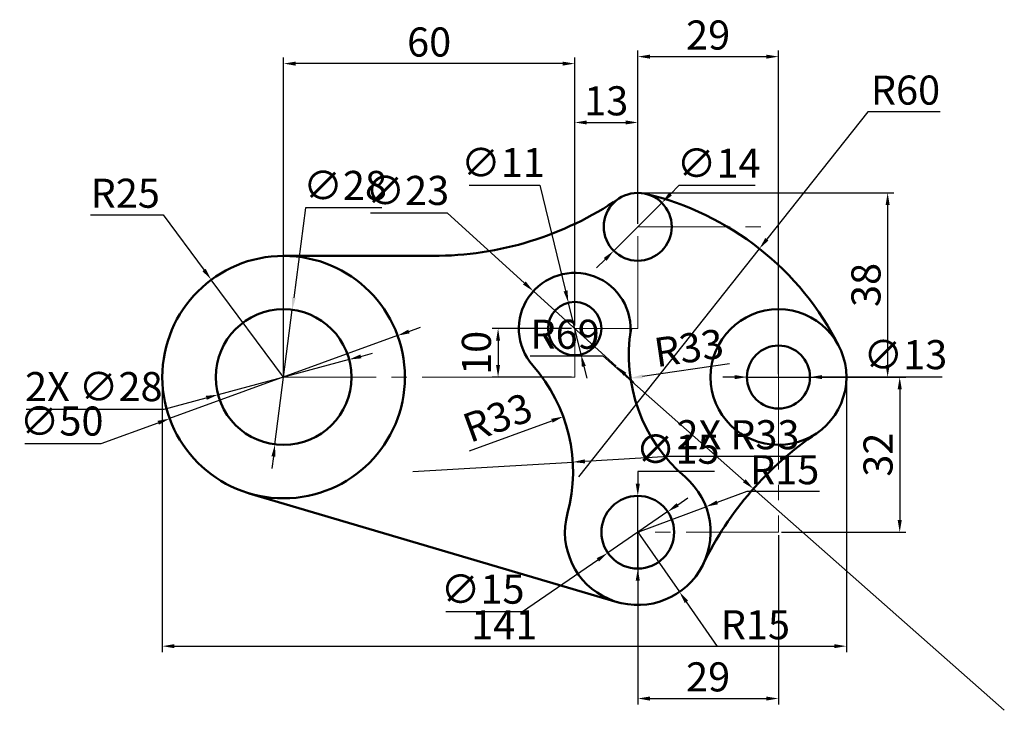
# Model space of a CAD drawing. Units: millimetres. Extents: x 48 to 251, y 61 to 204.
import ezdxf

# ---------------------------------------------------------------- set-up
doc = ezdxf.new("R2010")
doc.units = ezdxf.units.MM
doc.linetypes.add('CENTER2', pattern=[28.575, 19.05, -3.175, 3.175, -3.175])
for name, color, linetype, lineweight in [('M-CNTR', 4, 'CENTER2', 18), ('M-DIMS', 2, 'Continuous', 25), ('M-OUTL', 7, 'Continuous', 50)]:
    doc.layers.add(name, color=color, linetype=linetype, lineweight=lineweight)
doc.styles.get("Standard").update_dxf_attribs({"font": 'arial.ttf'})
doc.dimstyles.new('ISO-25', dxfattribs={"dimtxt": 6, "dimasz": 2.5, "dimexe": 1.25, "dimexo": 0.625, "dimtad": 1, "dimtoh": 1, "dimdec": 0, "dimtxsty": 'Standard', "dimcen": 2.5, "dimadec": 0, "dimazin": 0, "dimtfac": 1, "dimtdec": 0, "dimtmove": 0, "dimatfit": 3, "dimfxl": 1, "dimarcsym": 0})

# ---------------------------------------------------------------- blocks, each defined once
blk = doc.blocks.new('*D1')
at = {"layer": 'Defpoints', "color": 0, "transparency": 16777216}
for p in [(162.88, 140.02), (147.09, 130.02), (162.88, 130.02)]:
    blk.add_point(p, dxfattribs=at)
at = {"layer": 'M-DIMS', "color": 0, "lineweight": -2, "transparency": 16777216}
for p, q in [((162.25, 140.02), (145.84, 140.02)), ((147.09, 137.52), (147.09, 132.52)), ((162.25, 130.02), (145.84, 130.02))]:
    blk.add_line(p, q, dxfattribs=at)
at = {"layer": 'M-DIMS', "color": 0, "transparency": 16777216}
for points in [[(146.67, 137.52), (147.5, 137.52), (147.09, 140.02)], [(146.67, 132.52), (147.5, 132.52), (147.09, 130.02)]]:
    blk.add_solid(points, dxfattribs=at)
at = {"layer": 'M-DIMS', "color": 0, "transparency": 16777216, "insert": (143.4, 135.02), "char_height": 6, "attachment_point": 5, "rotation": 90}
blk.add_mtext('10', dxfattribs=at)
blk = doc.blocks.new('*D2')
at = {"layer": 'Defpoints', "color": 0, "transparency": 16777216}
for p in [(154.36, 147.74), (171.4, 132.29)]:
    blk.add_point(p, dxfattribs=at)
at = {"layer": 'M-DIMS', "color": 0, "lineweight": -2, "transparency": 16777216}
for p, q in [((120.81, 163.89), (136.56, 163.89)), ((136.56, 163.89), (152.51, 149.42)), ((171.4, 132.29), (154.36, 147.74)), ((173.25, 130.61), (175.1, 128.93))]:
    blk.add_line(p, q, dxfattribs=at)
at = {"layer": 'M-DIMS', "color": 0, "transparency": 16777216}
for points in [[(152.79, 149.73), (152.23, 149.11), (154.36, 147.74)], [(173.53, 130.92), (172.97, 130.3), (171.4, 132.29)]]:
    blk.add_solid(points, dxfattribs=at)
at = {"layer": 'M-DIMS', "color": 0, "transparency": 16777216, "insert": (128.37, 167.74), "char_height": 6, "attachment_point": 5}
blk.add_mtext('∅23', dxfattribs=at)
blk = doc.blocks.new('*D3')
at = {"layer": 'Defpoints', "color": 0, "transparency": 16777216}
for p in [(161.58, 145.36), (164.18, 134.67)]:
    blk.add_point(p, dxfattribs=at)
at = {"layer": 'M-DIMS', "color": 0, "lineweight": -2, "transparency": 16777216}
for p, q in [((141.11, 169.62), (155.7, 169.62)), ((155.7, 169.62), (160.99, 147.79)), ((164.18, 134.67), (161.58, 145.36)), ((164.77, 132.24), (165.35, 129.81))]:
    blk.add_line(p, q, dxfattribs=at)
at = {"layer": 'M-DIMS', "color": 0, "transparency": 16777216}
for points in [[(161.4, 147.89), (160.59, 147.69), (161.58, 145.36)], [(165.17, 132.34), (164.36, 132.14), (164.18, 134.67)]]:
    blk.add_solid(points, dxfattribs=at)
at = {"layer": 'M-DIMS', "color": 0, "transparency": 16777216, "insert": (148.09, 173.48), "char_height": 6, "attachment_point": 5}
blk.add_mtext('∅11', dxfattribs=at)
blk = doc.blocks.new('*D4')
at = {"layer": 'Defpoints', "color": 0, "transparency": 16777216}
for p in [(175.88, 182.53), (175.88, 161.02), (162.88, 140.02)]:
    blk.add_point(p, dxfattribs=at)
at = {"layer": 'M-DIMS', "color": 0, "lineweight": -2, "transparency": 16777216}
for p, q in [((162.88, 140.64), (162.88, 183.78)), ((175.88, 161.64), (175.88, 183.78)), ((165.38, 182.53), (173.38, 182.53))]:
    blk.add_line(p, q, dxfattribs=at)
at = {"layer": 'M-DIMS', "color": 0, "transparency": 16777216}
for points in [[(165.38, 182.95), (165.38, 182.12), (162.88, 182.53)], [(173.38, 182.95), (173.38, 182.12), (175.88, 182.53)]]:
    blk.add_solid(points, dxfattribs=at)
at = {"layer": 'M-DIMS', "color": 0, "transparency": 16777216, "insert": (169.38, 186.22), "char_height": 6, "attachment_point": 5}
blk.add_mtext('13', dxfattribs=at)
blk = doc.blocks.new('*D5')
at = {"layer": 'Defpoints', "color": 0, "transparency": 16777216}
for p in [(204.88, 130.02), (204.88, 98.02), (229.87, 98.02)]:
    blk.add_point(p, dxfattribs=at)
at = {"layer": 'M-DIMS', "color": 0, "lineweight": -2, "transparency": 16777216}
for p, q in [((205.5, 130.02), (231.12, 130.02)), ((229.87, 127.52), (229.87, 100.52)), ((205.5, 98.02), (231.12, 98.02))]:
    blk.add_line(p, q, dxfattribs=at)
at = {"layer": 'M-DIMS', "color": 0, "transparency": 16777216}
for points in [[(229.45, 127.52), (230.29, 127.52), (229.87, 130.02)], [(229.45, 100.52), (230.29, 100.52), (229.87, 98.02)]]:
    blk.add_solid(points, dxfattribs=at)
at = {"layer": 'M-DIMS', "color": 0, "transparency": 16777216, "insert": (226.18, 114.02), "char_height": 6, "attachment_point": 5, "rotation": 90}
blk.add_mtext('32', dxfattribs=at)
blk = doc.blocks.new('*D6')
at = {"layer": 'Defpoints', "color": 0, "transparency": 16777216}
for p in [(175.88, 98.02), (204.88, 98.02), (204.88, 63.73)]:
    blk.add_point(p, dxfattribs=at)
at = {"layer": 'M-DIMS', "color": 0, "lineweight": -2, "transparency": 16777216}
for p, q in [((175.88, 97.39), (175.88, 62.48)), ((204.88, 97.39), (204.88, 62.48)), ((178.38, 63.73), (202.38, 63.73))]:
    blk.add_line(p, q, dxfattribs=at)
at = {"layer": 'M-DIMS', "color": 0, "transparency": 16777216}
for points in [[(178.38, 64.14), (178.38, 63.31), (175.88, 63.73)], [(202.38, 64.14), (202.38, 63.31), (204.88, 63.73)]]:
    blk.add_solid(points, dxfattribs=at)
at = {"layer": 'M-DIMS', "color": 0, "transparency": 16777216, "insert": (190.38, 67.42), "char_height": 6, "attachment_point": 5}
blk.add_mtext('29', dxfattribs=at)
blk = doc.blocks.new('*D7')
at = {"layer": 'Defpoints', "color": 0, "transparency": 16777216}
for p in [(182.06, 102.27), (169.7, 93.76)]:
    blk.add_point(p, dxfattribs=at)
at = {"layer": 'M-DIMS', "color": 0, "lineweight": -2, "transparency": 16777216}
for p, q in [((184.12, 103.69), (186.18, 105.11)), ((182.06, 102.27), (169.7, 93.76)), ((152.11, 81.66), (167.64, 92.35)), ((136.32, 81.66), (152.11, 81.66))]:
    blk.add_line(p, q, dxfattribs=at)
at = {"layer": 'M-DIMS', "color": 0, "transparency": 16777216}
for points in [[(183.88, 104.03), (184.35, 103.34), (182.06, 102.27)], [(167.41, 92.69), (167.88, 92), (169.7, 93.76)]]:
    blk.add_solid(points, dxfattribs=at)
at = {"layer": 'M-DIMS', "color": 0, "transparency": 16777216, "insert": (143.9, 85.51), "char_height": 6, "attachment_point": 5}
blk.add_mtext('∅15', dxfattribs=at)
blk = doc.blocks.new('*D8')
at = {"layer": 'Defpoints', "color": 0, "transparency": 16777216}
for p in [(175.88, 98.02), (184.47, 85.72)]:
    blk.add_point(p, dxfattribs=at)
at = {"layer": 'M-DIMS', "color": 0, "lineweight": -2, "transparency": 16777216}
for p, q in [((175.88, 98.02), (184.47, 85.72)), ((192.31, 74.48), (185.9, 83.67)), ((207.31, 74.48), (192.31, 74.48))]:
    blk.add_line(p, q, dxfattribs=at)
at = {"layer": 'M-DIMS', "color": 0, "transparency": 16777216}
blk.add_solid([(186.24, 83.91), (185.56, 83.43), (184.47, 85.72)], dxfattribs=at)
at = {"layer": 'M-DIMS', "color": 0, "transparency": 16777216, "insert": (200.12, 78.17), "char_height": 6, "attachment_point": 5}
blk.add_mtext('R15', dxfattribs=at)
blk = doc.blocks.new('*D9')
at = {"layer": 'Defpoints', "color": 0, "transparency": 16777216}
for p in [(204.88, 196.11), (175.88, 161.02), (204.88, 130.02)]:
    blk.add_point(p, dxfattribs=at)
at = {"layer": 'M-DIMS', "color": 0, "lineweight": -2, "transparency": 16777216}
for p, q in [((175.88, 161.64), (175.88, 197.36)), ((204.88, 130.64), (204.88, 197.36)), ((178.38, 196.11), (202.38, 196.11))]:
    blk.add_line(p, q, dxfattribs=at)
at = {"layer": 'M-DIMS', "color": 0, "transparency": 16777216}
for points in [[(178.38, 196.52), (178.38, 195.69), (175.88, 196.11)], [(202.38, 196.52), (202.38, 195.69), (204.88, 196.11)]]:
    blk.add_solid(points, dxfattribs=at)
at = {"layer": 'M-DIMS', "color": 0, "transparency": 16777216, "insert": (190.38, 199.79), "char_height": 6, "attachment_point": 5}
blk.add_mtext('29', dxfattribs=at)
blk = doc.blocks.new('*D10')
at = {"layer": 'Defpoints', "color": 0, "transparency": 16777216}
for p in [(102.88, 194.67), (162.88, 140.02), (102.88, 130.02)]:
    blk.add_point(p, dxfattribs=at)
at = {"layer": 'M-DIMS', "color": 0, "lineweight": -2, "transparency": 16777216}
for p, q in [((102.88, 130.64), (102.88, 195.92)), ((162.88, 140.64), (162.88, 195.92)), ((160.38, 194.67), (105.38, 194.67))]:
    blk.add_line(p, q, dxfattribs=at)
at = {"layer": 'M-DIMS', "color": 0, "transparency": 16777216}
for points in [[(105.38, 195.08), (105.38, 194.25), (102.88, 194.67)], [(160.38, 195.08), (160.38, 194.25), (162.88, 194.67)]]:
    blk.add_solid(points, dxfattribs=at)
at = {"layer": 'M-DIMS', "color": 0, "transparency": 16777216, "insert": (132.88, 198.35), "char_height": 6, "attachment_point": 5}
blk.add_mtext('60', dxfattribs=at)
blk = doc.blocks.new('*D11')
at = {"layer": 'Defpoints', "color": 0, "transparency": 16777216}
for p in [(87.98, 150.09), (102.88, 130.02)]:
    blk.add_point(p, dxfattribs=at)
at = {"layer": 'M-DIMS', "color": 0, "lineweight": -2, "transparency": 16777216}
for p, q in [((63.05, 163.47), (78.06, 163.47)), ((78.06, 163.47), (86.49, 152.1)), ((102.88, 130.02), (87.98, 150.09))]:
    blk.add_line(p, q, dxfattribs=at)
at = {"layer": 'M-DIMS', "color": 0, "transparency": 16777216}
blk.add_solid([(86.83, 152.35), (86.16, 151.85), (87.98, 150.09)], dxfattribs=at)
at = {"layer": 'M-DIMS', "color": 0, "transparency": 16777216, "insert": (70.24, 167.16), "char_height": 6, "attachment_point": 5}
blk.add_mtext('R25', dxfattribs=at)
blk = doc.blocks.new('*D12')
at = {"layer": 'Defpoints', "color": 0, "transparency": 16777216}
for p in [(104.66, 143.9), (101.1, 116.13)]:
    blk.add_point(p, dxfattribs=at)
at = {"layer": 'M-DIMS', "color": 0, "lineweight": -2, "transparency": 16777216}
for p, q in [((107.36, 164.91), (104.98, 146.38)), ((123.12, 164.91), (107.36, 164.91)), ((101.1, 116.13), (104.66, 143.9)), ((100.78, 113.65), (100.46, 111.17))]:
    blk.add_line(p, q, dxfattribs=at)
at = {"layer": 'M-DIMS', "color": 0, "transparency": 16777216}
for points in [[(104.57, 146.44), (105.39, 146.33), (104.66, 143.9)], [(100.37, 113.7), (101.19, 113.6), (101.1, 116.13)]]:
    blk.add_solid(points, dxfattribs=at)
at = {"layer": 'M-DIMS', "color": 0, "transparency": 16777216, "insert": (115.55, 168.77), "char_height": 6, "attachment_point": 5}
blk.add_mtext('∅28', dxfattribs=at)
blk = doc.blocks.new('*D13')
at = {"layer": 'Defpoints', "color": 0, "transparency": 16777216}
for p in [(160.53, 121.88), (129.54, 110.54)]:
    blk.add_point(p, dxfattribs=at)
at = {"layer": 'M-DIMS', "color": 0, "lineweight": -2, "transparency": 16777216}
blk.add_line((141.2, 114.81), (158.19, 121.02), dxfattribs=at)
at = {"layer": 'M-DIMS', "color": 0, "transparency": 16777216}
blk.add_solid([(158.04, 121.41), (158.33, 120.63), (160.53, 121.88)], dxfattribs=at)
at = {"layer": 'M-DIMS', "color": 0, "transparency": 16777216, "insert": (147.25, 120.95), "char_height": 6, "attachment_point": 5, "rotation": 20.0942}
blk.add_mtext('R33', dxfattribs=at)
blk = doc.blocks.new('*D14')
at = {"layer": 'Defpoints', "color": 0, "transparency": 16777216}
for p in [(207.04, 134.53), (174.38, 129.79)]:
    blk.add_point(p, dxfattribs=at)
at = {"layer": 'M-DIMS', "color": 0, "lineweight": -2, "transparency": 16777216}
blk.add_line((194.76, 132.75), (176.86, 130.15), dxfattribs=at)
at = {"layer": 'M-DIMS', "color": 0, "transparency": 16777216}
blk.add_solid([(176.8, 130.57), (176.92, 129.74), (174.38, 129.79)], dxfattribs=at)
at = {"layer": 'M-DIMS', "color": 0, "transparency": 16777216, "insert": (186.51, 135.28), "char_height": 6, "attachment_point": 5, "rotation": 8.2467}
blk.add_mtext('R33', dxfattribs=at)
blk = doc.blocks.new('*D15')
at = {"layer": 'Defpoints', "color": 0, "transparency": 16777216}
for p in [(77.88, 130.02), (218.88, 130.02), (218.88, 74.53)]:
    blk.add_point(p, dxfattribs=at)
at = {"layer": 'M-DIMS', "color": 0, "lineweight": -2, "transparency": 16777216}
for p, q in [((77.88, 129.39), (77.88, 73.28)), ((218.88, 129.39), (218.88, 73.28)), ((80.38, 74.53), (216.38, 74.53))]:
    blk.add_line(p, q, dxfattribs=at)
at = {"layer": 'M-DIMS', "color": 0, "transparency": 16777216}
for points in [[(80.38, 74.95), (80.38, 74.12), (77.88, 74.53)], [(216.38, 74.95), (216.38, 74.12), (218.88, 74.53)]]:
    blk.add_solid(points, dxfattribs=at)
at = {"layer": 'M-DIMS', "color": 0, "transparency": 16777216, "insert": (148.38, 78.17), "char_height": 6, "attachment_point": 5}
blk.add_mtext('141', dxfattribs=at)
blk = doc.blocks.new('*D16')
at = {"layer": 'Defpoints', "color": 0, "transparency": 16777216}
for p in [(175.88, 168.02), (218.88, 130.02), (227.38, 130.02)]:
    blk.add_point(p, dxfattribs=at)
at = {"layer": 'M-DIMS', "color": 0, "lineweight": -2, "transparency": 16777216}
for p, q in [((176.5, 168.02), (228.63, 168.02)), ((227.38, 165.52), (227.38, 132.52)), ((219.5, 130.02), (228.63, 130.02))]:
    blk.add_line(p, q, dxfattribs=at)
at = {"layer": 'M-DIMS', "color": 0, "transparency": 16777216}
for points in [[(226.96, 165.52), (227.8, 165.52), (227.38, 168.02)], [(226.96, 132.52), (227.8, 132.52), (227.38, 130.02)]]:
    blk.add_solid(points, dxfattribs=at)
at = {"layer": 'M-DIMS', "color": 0, "transparency": 16777216, "insert": (223.69, 149.02), "char_height": 6, "attachment_point": 5, "rotation": 90}
blk.add_mtext('38', dxfattribs=at)
blk = doc.blocks.new('*D17')
at = {"layer": 'Defpoints', "color": 0, "transparency": 16777216}
for p in [(200.95, 156.5), (163.75, 109.42)]:
    blk.add_point(p, dxfattribs=at)
at = {"layer": 'M-DIMS', "color": 0, "lineweight": -2, "transparency": 16777216}
for p, q in [((223.27, 184.74), (202.5, 158.46)), ((238.21, 184.74), (223.27, 184.74)), ((163.75, 109.42), (200.95, 156.5))]:
    blk.add_line(p, q, dxfattribs=at)
at = {"layer": 'M-DIMS', "color": 0, "transparency": 16777216}
blk.add_solid([(202.17, 158.72), (202.83, 158.2), (200.95, 156.5)], dxfattribs=at)
at = {"layer": 'M-DIMS', "color": 0, "transparency": 16777216, "insert": (231.06, 188.43), "char_height": 6, "attachment_point": 5}
blk.add_mtext('R60', dxfattribs=at)
blk = doc.blocks.new('*D18')
at = {"layer": 'Defpoints', "color": 0, "transparency": 16777216}
for p in [(199.72, 106.98), (251.43, 61.3)]:
    blk.add_point(p, dxfattribs=at)
at = {"layer": 'M-DIMS', "color": 0, "lineweight": -2, "transparency": 16777216}
for p, q in [((153.71, 134.39), (168.69, 134.39)), ((168.69, 134.39), (197.84, 108.63)), ((251.43, 61.3), (199.72, 106.98))]:
    blk.add_line(p, q, dxfattribs=at)
at = {"layer": 'M-DIMS', "color": 0, "transparency": 16777216}
blk.add_solid([(198.12, 108.95), (197.57, 108.32), (199.72, 106.98)], dxfattribs=at)
at = {"layer": 'M-DIMS', "color": 0, "transparency": 16777216, "insert": (160.89, 138.08), "char_height": 6, "attachment_point": 5}
blk.add_mtext('R69', dxfattribs=at)
blk = doc.blocks.new('*D19')
at = {"layer": 'Defpoints', "color": 0, "transparency": 16777216}
for p in [(162.48, 112.5), (129.54, 110.54)]:
    blk.add_point(p, dxfattribs=at)
at = {"layer": 'M-DIMS', "color": 0, "lineweight": -2, "transparency": 16777216}
for p, q in [((182.25, 113.67), (164.98, 112.64)), ((210.21, 113.67), (182.25, 113.67)), ((129.54, 110.54), (162.48, 112.5))]:
    blk.add_line(p, q, dxfattribs=at)
at = {"layer": 'M-DIMS', "color": 0, "transparency": 16777216}
blk.add_solid([(164.96, 113.06), (165, 112.23), (162.48, 112.5)], dxfattribs=at)
at = {"layer": 'M-DIMS', "color": 0, "transparency": 16777216, "insert": (196.54, 117.36), "char_height": 6, "attachment_point": 5}
blk.add_mtext('2X R33', dxfattribs=at)
blk = doc.blocks.new('*D20')
at = {"layer": 'Defpoints', "color": 0, "transparency": 16777216}
for p in [(126.37, 138.57), (79.39, 121.46)]:
    blk.add_point(p, dxfattribs=at)
at = {"layer": 'M-DIMS', "color": 0, "lineweight": -2, "transparency": 16777216}
for p, q in [((128.72, 139.43), (131.07, 140.29)), ((126.37, 138.57), (79.39, 121.46)), ((65.3, 116.33), (77.04, 120.6)), ((49.57, 116.33), (65.3, 116.33))]:
    blk.add_line(p, q, dxfattribs=at)
at = {"layer": 'M-DIMS', "color": 0, "transparency": 16777216}
for points in [[(128.58, 139.82), (128.86, 139.04), (126.37, 138.57)], [(76.9, 121), (77.18, 120.21), (79.39, 121.46)]]:
    blk.add_solid(points, dxfattribs=at)
at = {"layer": 'M-DIMS', "color": 0, "transparency": 16777216, "insert": (57.12, 120.18), "char_height": 6, "attachment_point": 5}
blk.add_mtext('∅50', dxfattribs=at)
blk = doc.blocks.new('*D21')
at = {"layer": 'Defpoints', "color": 0, "transparency": 16777216}
for p in [(189.92, 103.29), (175.88, 98.02)]:
    blk.add_point(p, dxfattribs=at)
at = {"layer": 'M-DIMS', "color": 0, "lineweight": -2, "transparency": 16777216}
for p, q in [((198.35, 106.46), (192.26, 104.17)), ((213.35, 106.46), (198.35, 106.46)), ((175.88, 98.02), (189.92, 103.29))]:
    blk.add_line(p, q, dxfattribs=at)
at = {"layer": 'M-DIMS', "color": 0, "transparency": 16777216}
blk.add_solid([(192.12, 104.56), (192.41, 103.78), (189.92, 103.29)], dxfattribs=at)
at = {"layer": 'M-DIMS', "color": 0, "transparency": 16777216, "insert": (206.16, 110.14), "char_height": 6, "attachment_point": 5}
blk.add_mtext('R15', dxfattribs=at)
blk = doc.blocks.new('*D22')
at = {"layer": 'Defpoints', "color": 0, "transparency": 16777216}
for p in [(116.4, 133.64), (89.36, 126.39)]:
    blk.add_point(p, dxfattribs=at)
at = {"layer": 'M-DIMS', "color": 0, "lineweight": -2, "transparency": 16777216}
for p, q in [((118.82, 134.29), (121.23, 134.94)), ((116.4, 133.64), (89.36, 126.39)), ((78.29, 123.43), (86.94, 125.75)), ((49.85, 123.43), (78.29, 123.43))]:
    blk.add_line(p, q, dxfattribs=at)
at = {"layer": 'M-DIMS', "color": 0, "transparency": 16777216}
for points in [[(118.71, 134.69), (118.93, 133.89), (116.4, 133.64)], [(86.83, 126.15), (87.05, 125.34), (89.36, 126.39)]]:
    blk.add_solid(points, dxfattribs=at)
at = {"layer": 'M-DIMS', "color": 0, "transparency": 16777216, "insert": (63.76, 127.28), "char_height": 6, "attachment_point": 5}
blk.add_mtext('2X ∅28', dxfattribs=at)
blk = doc.blocks.new('*D23')
at = {"layer": 'Defpoints', "color": 0, "transparency": 16777216}
for p in [(175.88, 105.52), (175.88, 90.52)]:
    blk.add_point(p, dxfattribs=at)
at = {"layer": 'M-DIMS', "color": 0, "lineweight": -2, "transparency": 16777216}
for p, q in [((191.67, 110.52), (175.88, 110.52)), ((175.88, 110.52), (175.88, 108.02)), ((175.88, 90.52), (175.88, 105.52)), ((175.88, 88.02), (175.88, 85.52))]:
    blk.add_line(p, q, dxfattribs=at)
at = {"layer": 'M-DIMS', "color": 0, "transparency": 16777216}
for points in [[(175.46, 108.02), (176.3, 108.02), (175.88, 105.52)], [(175.46, 88.02), (176.3, 88.02), (175.88, 90.52)]]:
    blk.add_solid(points, dxfattribs=at)
at = {"layer": 'M-DIMS', "color": 0, "transparency": 16777216, "insert": (184.09, 114.37), "char_height": 6, "attachment_point": 5}
blk.add_mtext('∅15', dxfattribs=at)
blk = doc.blocks.new('*D24')
at = {"layer": 'Defpoints', "color": 0, "transparency": 16777216}
for p in [(180.83, 165.97), (170.93, 156.07)]:
    blk.add_point(p, dxfattribs=at)
at = {"layer": 'M-DIMS', "color": 0, "lineweight": -2, "transparency": 16777216}
for p, q in [((184.36, 169.5), (182.6, 167.74)), ((200.09, 169.5), (184.36, 169.5)), ((170.93, 156.07), (180.83, 165.97)), ((169.16, 154.3), (167.4, 152.53))]:
    blk.add_line(p, q, dxfattribs=at)
at = {"layer": 'M-DIMS', "color": 0, "transparency": 16777216}
for points in [[(182.3, 168.03), (182.89, 167.44), (180.83, 165.97)], [(168.87, 154.59), (169.46, 154), (170.93, 156.07)]]:
    blk.add_solid(points, dxfattribs=at)
at = {"layer": 'M-DIMS', "color": 0, "transparency": 16777216, "insert": (192.54, 173.36), "char_height": 6, "attachment_point": 5}
blk.add_mtext('∅14', dxfattribs=at)
blk = doc.blocks.new('*D25')
at = {"layer": 'Defpoints', "color": 0, "transparency": 16777216}
for p in [(198.38, 130.02), (211.38, 130.02)]:
    blk.add_point(p, dxfattribs=at)
at = {"layer": 'M-DIMS', "color": 0, "lineweight": -2, "transparency": 16777216}
for p, q in [((195.88, 130.02), (193.38, 130.02)), ((198.38, 130.02), (211.38, 130.02)), ((222.84, 130.02), (213.88, 130.02)), ((238.59, 130.02), (222.84, 130.02))]:
    blk.add_line(p, q, dxfattribs=at)
at = {"layer": 'M-DIMS', "color": 0, "transparency": 16777216}
for points in [[(195.88, 130.43), (195.88, 129.6), (198.38, 130.02)], [(213.88, 130.43), (213.88, 129.6), (211.38, 130.02)]]:
    blk.add_solid(points, dxfattribs=at)
at = {"layer": 'M-DIMS', "color": 0, "transparency": 16777216, "insert": (231.03, 133.87), "char_height": 6, "attachment_point": 5}
blk.add_mtext('∅13', dxfattribs=at)

msp = doc.modelspace()

# ---------------------------------------------------------------- linework, layer by layer
at = {"layer": 'M-CNTR'}
msp.add_lwpolyline([(102.88, 130.02), (162.88, 130.02), (162.88, 140.02), (175.88, 140.02), (175.88, 161.02), (204.88, 161.02), (204.88, 130.02), (204.88, 98.02), (175.88, 98.02)], dxfattribs=at)
at = {"layer": 'M-OUTL'}
msp.add_line((95.8, 106.04), (171.63, 83.63), dxfattribs=at)
for points in [[(102.88, 155.02), (133.68, 155.02, 0.150531), (171.94, 166.8)], [(174.5, 140.02, 0.263725), (185.62, 109.43, -1.816079), (161.4, 101.93, 0.252141), (154.26, 132.4, -1.548254), (174.29, 138.6)]]:
    msp.add_lwpolyline(points, format="xyb", dxfattribs=at)
for centre, radius in [((175.88, 161.02), 7), ((102.88, 130.02), 25), ((162.88, 140.02), 5.5), ((102.88, 130.02), 14), ((204.88, 130.02), 14), ((204.88, 130.02), 6.5), ((175.88, 98.02), 7.5)]:
    msp.add_circle(centre, radius, dxfattribs=at)
for centre, radius, start, end in [((163.75, 109.42), 60, 26.5938, 76.7659), ((251.43, 61.3), 69, 124.1143, 154.0803)]:
    msp.add_arc(centre, radius, start, end, dxfattribs=at)

# ---------------------------------------------------------------- dimensions: what is measured, and where the dimension line sits
at = {"layer": 'M-DIMS'}
for base, p1, p2, override, picture, middle in [((204.88, 196.11), (175.88, 161.02), (204.88, 130.02), {"dimclrd": 0, "dimclre": 0, "dimclrt": 0}, '*D9', (190.38, 199.79)), ((102.88, 194.67), (162.88, 140.02), (102.88, 130.02), {"dimclrd": 0, "dimclre": 0, "dimclrt": 0}, '*D10', (132.88, 198.35)), ((175.88, 182.53), (162.88, 140.02), (175.88, 161.02), {"dimclrd": 0, "dimclre": 0, "dimclrt": 0}, '*D4', (169.38, 186.22)), ((218.88, 74.53), (77.88, 130.02), (218.88, 130.02), {"dimdec": 0, "dimlfac": 1, "dimrnd": 0, "dimzin": 0, "dimdsep": 46, "dimlunit": 2}, '*D15', (148.38, 78.17)), ((204.88, 63.73), (175.88, 98.02), (204.88, 98.02), {"dimclrd": 0, "dimclre": 0, "dimclrt": 0}, '*D6', (190.38, 67.42))]:
    dim = msp.add_linear_dim(base=base, p1=p1, p2=p2, dimstyle='ISO-25', override=override, dxfattribs=at)
    dim.commit()
    dim.dimension.update_dxf_attribs({"geometry": picture, "text_midpoint": middle})
for center, mpoint, override, picture, middle in [((163.75, 109.42), (200.95, 156.5), {"dimdec": 0, "dimlfac": 1, "dimrnd": 0, "dimzin": 0, "dimdsep": 46, "dimlunit": 2}, '*D17', (231.06, 184.74)), ((102.88, 130.02), (87.98, 150.09), {"dimclrd": 0, "dimclre": 0, "dimclrt": 0}, '*D11', (70.24, 163.47)), ((251.43, 61.3), (199.72, 106.98), {"dimdec": 0, "dimlfac": 1, "dimrnd": 0, "dimzin": 0, "dimdsep": 46, "dimlunit": 2}, '*D18', (160.89, 134.39)), ((207.04, 134.53), (174.38, 129.79), {"dimclrd": 0, "dimclre": 0, "dimclrt": 0}, '*D14', (187.04, 131.63)), ((129.54, 110.54), (160.53, 121.88), {"dimclrd": 0, "dimclre": 0, "dimclrt": 0}, '*D13', (148.52, 117.48)), ((175.88, 98.02), (189.92, 103.29), {"dimdec": 0, "dimlfac": 1, "dimrnd": 0, "dimzin": 0, "dimdsep": 46, "dimlunit": 2}, '*D21', (206.16, 106.46)), ((175.88, 98.02), (184.47, 85.72), {"dimclrd": 0, "dimclre": 0, "dimclrt": 0}, '*D8', (200.12, 74.48))]:
    dim = msp.add_radius_dim(center=center, mpoint=mpoint, dimstyle='ISO-25', override=override, dxfattribs=at)
    dim.commit()
    dim.dimension.update_dxf_attribs({"geometry": picture, "text_midpoint": middle, "dimtype": 164})
for p1, p2, override, picture, middle in [((164.18, 134.67), (161.58, 145.36), {"dimclrd": 0, "dimclre": 0, "dimclrt": 0}, '*D3', (148.09, 169.62)), ((170.93, 156.07), (180.83, 165.97), {"dimdec": 0, "dimlfac": 1, "dimrnd": 0, "dimzin": 0, "dimdsep": 46, "dimlunit": 2}, '*D24', (192.54, 169.5)), ((101.1, 116.13), (104.66, 143.9), {"dimclrd": 0, "dimclre": 0, "dimclrt": 0}, '*D12', (115.55, 164.91)), ((171.4, 132.29), (154.36, 147.74), {"dimclrd": 0, "dimclre": 0, "dimclrt": 0}, '*D2', (128.37, 163.89)), ((126.37, 138.57), (79.39, 121.46), {"dimdec": 0, "dimlfac": 1, "dimrnd": 0, "dimzin": 0, "dimdsep": 46, "dimlunit": 2}, '*D20', (57.12, 116.33)), ((198.38, 130.02), (211.38, 130.02), {"dimdec": 0, "dimlfac": 1, "dimrnd": 0, "dimzin": 0, "dimdsep": 46, "dimlunit": 2}, '*D25', (222.84, 130.02)), ((175.88, 90.52), (175.88, 105.52), {"dimdec": 0, "dimlfac": 1, "dimrnd": 0, "dimzin": 0, "dimdsep": 46, "dimlunit": 2}, '*D23', (184.09, 110.52)), ((182.06, 102.27), (169.7, 93.76), {"dimclrd": 0, "dimclre": 0, "dimclrt": 0}, '*D7', (143.9, 81.66))]:
    dim = msp.add_diameter_dim_2p(p1=p1, p2=p2, dimstyle='ISO-25', override=override, dxfattribs=at)
    dim.commit()
    dim.dimension.update_dxf_attribs({"geometry": picture, "text_midpoint": middle, "dimtype": 163})
for base, p1, p2, override, picture, middle in [((227.38, 130.02), (175.88, 168.02), (218.88, 130.02), {"dimdec": 0, "dimlfac": 1, "dimrnd": 0, "dimzin": 0, "dimdsep": 46, "dimlunit": 2}, '*D16', (223.69, 149.02)), ((147.09, 130.02), (162.88, 140.02), (162.88, 130.02), {"dimclrd": 0, "dimclre": 0, "dimclrt": 0}, '*D1', (143.4, 135.02)), ((229.87, 98.02), (204.88, 130.02), (204.88, 98.02), {"dimclrd": 0, "dimclre": 0, "dimclrt": 0}, '*D5', (226.18, 114.02))]:
    dim = msp.add_linear_dim(base=base, p1=p1, p2=p2, angle=90, dimstyle='ISO-25', override=override, dxfattribs=at)
    dim.commit()
    dim.dimension.update_dxf_attribs({"geometry": picture, "text_midpoint": middle})
dim = msp.add_diameter_dim_2p(p1=(116.4, 133.64), p2=(89.36, 126.39), text='2X <>', dimstyle='ISO-25', override={"dimdec": 0, "dimlfac": 1, "dimrnd": 0, "dimzin": 0, "dimdsep": 46, "dimlunit": 2}, dxfattribs=at)
dim.commit()
dim.dimension.update_dxf_attribs({"geometry": '*D22', "text_midpoint": (63.76, 123.43), "dimtype": 163})
dim = msp.add_radius_dim(center=(129.54, 110.54), mpoint=(162.48, 112.5), text='2X <>', dimstyle='ISO-25', override={"dimdec": 0, "dimlfac": 1, "dimrnd": 0, "dimzin": 0, "dimdsep": 46, "dimlunit": 2}, dxfattribs=at)
dim.commit()
dim.dimension.update_dxf_attribs({"geometry": '*D19', "text_midpoint": (182.25, 113.67), "dimtype": 164})

doc.saveas('drawing.dxf')
